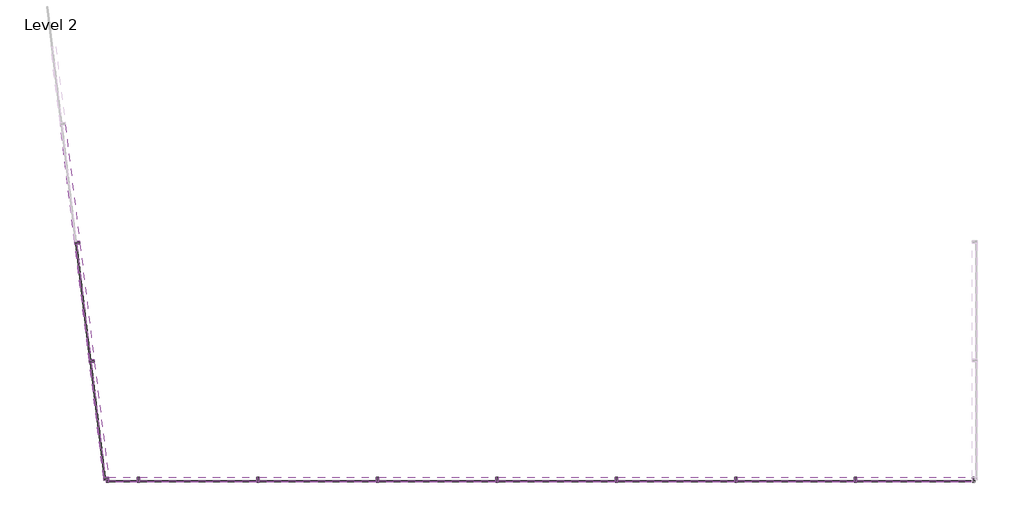
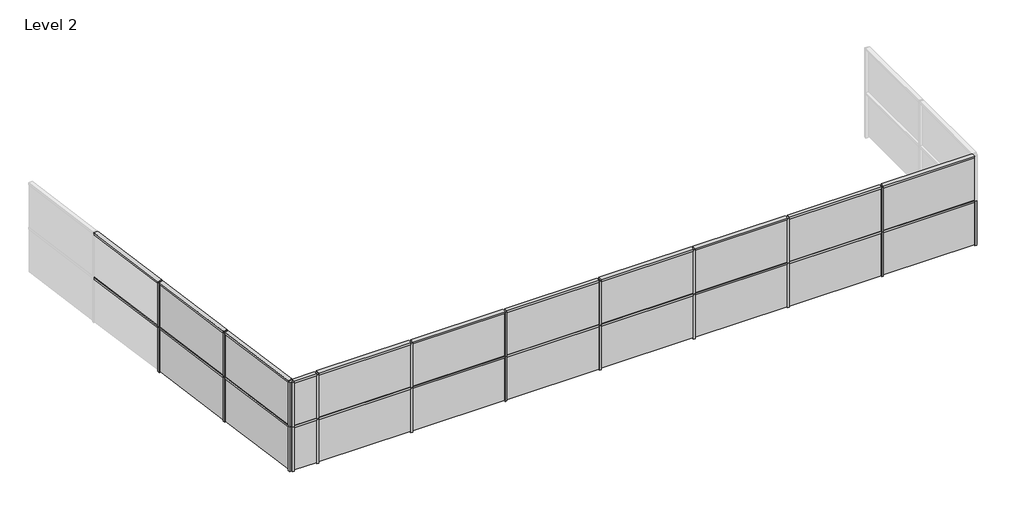
# One storey, part 1 of 2: 45 members, 20 plates.
"""IFC4 building model written with IfcOpenShell, lengths in millimetres."""

from ifc_helpers import new_model, si_unit, origin, place, context, project, spatial, transform, mapped, element, save
from components import member_19d0a4ec, member_8cef0660, member_82905deb, member_4491d118, member_0c11e56c, system_panel_glazed_e46d4b42, system_panel_glazed_2a6c68b7, system_panel_glazed_9d0e0944

model = new_model("IFC4")

# Units and contexts
model_context = context("Model", 3, world=origin())
ifc_project = project(units=[si_unit("LENGTHUNIT", "METRE", prefix="MILLI")], contexts=[model_context])

# Site, building, storey
site = spatial("IfcSite", under=ifc_project)
building = spatial("IfcBuilding", under=site)
storey = spatial("IfcBuildingStorey", under=building, Name="Level 2", Elevation=3048.0)

# Members
placement = place(None, origin())
member_shape = member_19d0a4ec(model_context)
element("IfcMember", 1, ObjectType="Rectangular Mullion : 2.5\" x 5\" rectangular", at=placement, inside=storey, context=model_context, shape_type="MappedRepresentation", body=[
    mapped(member_shape, transform((-8260.4765148, -6916.1096898, 4572.0), x_axis=(0.0, 0.0, 1.0), y_axis=(-0.9925461516413222, -0.12186934340514591, 0.0), z_axis=(0.12186934340514591, -0.9925461516413222, 0.0))),
])
element("IfcMember", 2, ObjectType="Rectangular Mullion : 2.5\" x 5\" rectangular", at=placement, inside=storey, context=model_context, shape_type="MappedRepresentation", body=[
    mapped(member_shape, transform((-8260.4765148, -6916.1096898, 6096.0), x_axis=(0.0, 0.0, 1.0), y_axis=(-0.9925461516413222, -0.12186934340514587, 0.0), z_axis=(0.12186934340514587, -0.9925461516413222, 0.0))),
])
element("IfcMember", 3, ObjectType="Rectangular Mullion : 2.5\" x 5\" rectangular", at=placement, inside=storey, context=model_context, shape_type="MappedRepresentation", body=[
    mapped(member_shape, transform((13839.0156363, -6979.1363705, 4572.0), x_axis=(0.0, 0.0, 1.0), y_axis=(0.0, -1.0, 0.0), z_axis=(1.0, 0.0, 0.0))),
])
element("IfcMember", 4, ObjectType="Rectangular Mullion : 2.5\" x 5\" rectangular", at=placement, inside=storey, context=model_context, shape_type="MappedRepresentation", body=[
    mapped(member_shape, transform((13839.0156363, -6979.1363705, 6096.0), x_axis=(0.0, 0.0, 1.0), y_axis=(0.0, -1.0, 0.0), z_axis=(1.0, 0.0, 0.0))),
])
member_2_shape = member_8cef0660(model_context)
element("IfcMember", 5, ObjectType="Rectangular Mullion : 2.5\" x 5\" rectangular", at=placement, inside=storey, context=model_context, shape_type="MappedRepresentation", body=[
    mapped(member_2_shape, transform((-8628.0649219, -3922.3423596, 4572.0), x_axis=(0.0, 0.0, 1.0), y_axis=(-0.9925461516413222, -0.12186934340514596, 0.0), z_axis=(0.12186934340514596, -0.9925461516413222, 0.0))),
])
element("IfcMember", 6, ObjectType="Rectangular Mullion : 2.5\" x 5\" rectangular", at=placement, inside=storey, context=model_context, shape_type="MappedRepresentation", body=[
    mapped(member_2_shape, transform((-8999.5226806, -897.0616894, 4572.0), x_axis=(0.0, 0.0, 1.0), y_axis=(-0.9925461516413222, -0.12186934340514602, 0.0), z_axis=(0.12186934340514602, -0.9925461516413222, 0.0))),
])
element("IfcMember", 7, ObjectType="Rectangular Mullion : 2.5\" x 5\" rectangular", at=placement, inside=storey, context=model_context, shape_type="MappedRepresentation", body=[
    mapped(member_2_shape, transform((-8628.0649219, -3922.3423596, 6096.0), x_axis=(0.0, 0.0, 1.0), y_axis=(-0.9925461516413222, -0.12186934340514596, 0.0), z_axis=(0.12186934340514596, -0.9925461516413222, 0.0))),
])
element("IfcMember", 8, ObjectType="Rectangular Mullion : 2.5\" x 5\" rectangular", at=placement, inside=storey, context=model_context, shape_type="MappedRepresentation", body=[
    mapped(member_2_shape, transform((-8999.5226806, -897.0616894, 6096.0), x_axis=(0.0, 0.0, 1.0), y_axis=(-0.9925461516413222, -0.12186934340514602, 0.0), z_axis=(0.12186934340514602, -0.9925461516413222, 0.0))),
])
element("IfcMember", 9, ObjectType="Rectangular Mullion : 2.5\" x 5\" rectangular", at=placement, inside=storey, context=model_context, shape_type="MappedRepresentation", body=[
    mapped(member_2_shape, transform((10822.765636, -6979.1363705, 4572.0), x_axis=(0.0, 0.0, 1.0), y_axis=(0.0, -1.0, 0.0), z_axis=(1.0, 0.0, 0.0))),
])
element("IfcMember", 10, ObjectType="Rectangular Mullion : 2.5\" x 5\" rectangular", at=placement, inside=storey, context=model_context, shape_type="MappedRepresentation", body=[
    mapped(member_2_shape, transform((7774.765636, -6979.1363705, 4572.0), x_axis=(0.0, 0.0, 1.0), y_axis=(0.0, -1.0, 0.0), z_axis=(1.0, 0.0, 0.0))),
])
element("IfcMember", 11, ObjectType="Rectangular Mullion : 2.5\" x 5\" rectangular", at=placement, inside=storey, context=model_context, shape_type="MappedRepresentation", body=[
    mapped(member_2_shape, transform((4726.765636, -6979.1363705, 4572.0), x_axis=(0.0, 0.0, 1.0), y_axis=(0.0, -1.0, 0.0), z_axis=(1.0, 0.0, 0.0))),
])
element("IfcMember", 12, ObjectType="Rectangular Mullion : 2.5\" x 5\" rectangular", at=placement, inside=storey, context=model_context, shape_type="MappedRepresentation", body=[
    mapped(member_2_shape, transform((1678.765636, -6979.1363705, 4572.0), x_axis=(0.0, 0.0, 1.0), y_axis=(0.0, -1.0, 0.0), z_axis=(1.0, 0.0, 0.0))),
])
element("IfcMember", 13, ObjectType="Rectangular Mullion : 2.5\" x 5\" rectangular", at=placement, inside=storey, context=model_context, shape_type="MappedRepresentation", body=[
    mapped(member_2_shape, transform((-1369.234364, -6979.1363705, 4572.0), x_axis=(0.0, 0.0, 1.0), y_axis=(0.0, -1.0, 0.0), z_axis=(1.0, 0.0, 0.0))),
])
element("IfcMember", 14, ObjectType="Rectangular Mullion : 2.5\" x 5\" rectangular", at=placement, inside=storey, context=model_context, shape_type="MappedRepresentation", body=[
    mapped(member_2_shape, transform((-4417.234364, -6979.1363705, 4572.0), x_axis=(0.0, 0.0, 1.0), y_axis=(0.0, -1.0, 0.0), z_axis=(1.0, 0.0, 0.0))),
])
element("IfcMember", 15, ObjectType="Rectangular Mullion : 2.5\" x 5\" rectangular", at=placement, inside=storey, context=model_context, shape_type="MappedRepresentation", body=[
    mapped(member_2_shape, transform((10822.765636, -6979.1363705, 6096.0), x_axis=(0.0, 0.0, 1.0), y_axis=(0.0, -1.0, 0.0), z_axis=(1.0, 0.0, 0.0))),
])
element("IfcMember", 16, ObjectType="Rectangular Mullion : 2.5\" x 5\" rectangular", at=placement, inside=storey, context=model_context, shape_type="MappedRepresentation", body=[
    mapped(member_2_shape, transform((7774.765636, -6979.1363705, 6096.0), x_axis=(0.0, 0.0, 1.0), y_axis=(0.0, -1.0, 0.0), z_axis=(1.0, 0.0, 0.0))),
])
element("IfcMember", 17, ObjectType="Rectangular Mullion : 2.5\" x 5\" rectangular", at=placement, inside=storey, context=model_context, shape_type="MappedRepresentation", body=[
    mapped(member_2_shape, transform((4726.765636, -6979.1363705, 6096.0), x_axis=(0.0, 0.0, 1.0), y_axis=(0.0, -1.0, 0.0), z_axis=(1.0, 0.0, 0.0))),
])
element("IfcMember", 18, ObjectType="Rectangular Mullion : 2.5\" x 5\" rectangular", at=placement, inside=storey, context=model_context, shape_type="MappedRepresentation", body=[
    mapped(member_2_shape, transform((1678.765636, -6979.1363705, 6096.0), x_axis=(0.0, 0.0, 1.0), y_axis=(0.0, -1.0, 0.0), z_axis=(1.0, 0.0, 0.0))),
])
element("IfcMember", 19, ObjectType="Rectangular Mullion : 2.5\" x 5\" rectangular", at=placement, inside=storey, context=model_context, shape_type="MappedRepresentation", body=[
    mapped(member_2_shape, transform((-1369.234364, -6979.1363705, 6096.0), x_axis=(0.0, 0.0, 1.0), y_axis=(0.0, -1.0, 0.0), z_axis=(1.0, 0.0, 0.0))),
])
element("IfcMember", 20, ObjectType="Rectangular Mullion : 2.5\" x 5\" rectangular", at=placement, inside=storey, context=model_context, shape_type="MappedRepresentation", body=[
    mapped(member_2_shape, transform((-4417.234364, -6979.1363705, 6096.0), x_axis=(0.0, 0.0, 1.0), y_axis=(0.0, -1.0, 0.0), z_axis=(1.0, 0.0, 0.0))),
])
member_3_shape = member_82905deb(model_context)
element("IfcMember", 21, ObjectType="Rectangular Mullion : 2.5\" x 5\" rectangular", at=placement, inside=storey, context=model_context, shape_type="MappedRepresentation", body=[
    mapped(member_3_shape, transform((-8624.1955702, -3953.8557, 4572.0), x_axis=(-0.12186934340514591, 0.9925461516413222, 0.0), y_axis=(-0.9925461516413222, -0.12186934340514591, 0.0), z_axis=(0.0, 0.0, 1.0))),
])
element("IfcMember", 22, ObjectType="Rectangular Mullion : 2.5\" x 5\" rectangular", at=placement, inside=storey, context=model_context, shape_type="MappedRepresentation", body=[
    mapped(member_3_shape, transform((-8624.1955702, -3953.8557, 6096.0), x_axis=(-0.12186934340514591, 0.9925461516413222, 0.0), y_axis=(-0.9925461516413222, -0.12186934340514591, 0.0), z_axis=(0.0, 0.0, 1.0))),
])
element("IfcMember", 23, ObjectType="Rectangular Mullion : 2.5\" x 5\" rectangular", at=placement, inside=storey, context=model_context, shape_type="MappedRepresentation", body=[
    mapped(member_3_shape, transform((-8995.6533289, -928.5750297, 4572.0), x_axis=(-0.12186934340514591, 0.9925461516413222, 0.0), y_axis=(-0.9925461516413222, -0.12186934340514591, 0.0), z_axis=(0.0, 0.0, 1.0))),
])
element("IfcMember", 24, ObjectType="Rectangular Mullion : 2.5\" x 5\" rectangular", at=placement, inside=storey, context=model_context, shape_type="MappedRepresentation", body=[
    mapped(member_3_shape, transform((-8995.6533289, -928.5750297, 6096.0), x_axis=(-0.12186934340514591, 0.9925461516413222, 0.0), y_axis=(-0.9925461516413222, -0.12186934340514591, 0.0), z_axis=(0.0, 0.0, 1.0))),
])
element("IfcMember", 25, ObjectType="Rectangular Mullion : 2.5\" x 5\" rectangular", at=placement, inside=storey, context=model_context, shape_type="MappedRepresentation", body=[
    mapped(member_3_shape, transform((10854.515636, -6979.1363705, 4572.0), x_axis=(-1.0, 0.0, 0.0), y_axis=(0.0, -1.0, 0.0), z_axis=(0.0, 0.0, 1.0))),
])
element("IfcMember", 26, ObjectType="Rectangular Mullion : 2.5\" x 5\" rectangular", at=placement, inside=storey, context=model_context, shape_type="MappedRepresentation", body=[
    mapped(member_3_shape, transform((10854.515636, -6979.1363705, 6096.0), x_axis=(-1.0, 0.0, 0.0), y_axis=(0.0, -1.0, 0.0), z_axis=(0.0, 0.0, 1.0))),
])
element("IfcMember", 27, ObjectType="Rectangular Mullion : 2.5\" x 5\" rectangular", at=placement, inside=storey, context=model_context, shape_type="MappedRepresentation", body=[
    mapped(member_3_shape, transform((7806.515636, -6979.1363705, 4572.0), x_axis=(-1.0, 0.0, 0.0), y_axis=(0.0, -1.0, 0.0), z_axis=(0.0, 0.0, 1.0))),
])
element("IfcMember", 28, ObjectType="Rectangular Mullion : 2.5\" x 5\" rectangular", at=placement, inside=storey, context=model_context, shape_type="MappedRepresentation", body=[
    mapped(member_3_shape, transform((7806.515636, -6979.1363705, 6096.0), x_axis=(-1.0, 0.0, 0.0), y_axis=(0.0, -1.0, 0.0), z_axis=(0.0, 0.0, 1.0))),
])
element("IfcMember", 29, ObjectType="Rectangular Mullion : 2.5\" x 5\" rectangular", at=placement, inside=storey, context=model_context, shape_type="MappedRepresentation", body=[
    mapped(member_3_shape, transform((4758.515636, -6979.1363705, 4572.0), x_axis=(-1.0, 0.0, 0.0), y_axis=(0.0, -1.0, 0.0), z_axis=(0.0, 0.0, 1.0))),
])
element("IfcMember", 30, ObjectType="Rectangular Mullion : 2.5\" x 5\" rectangular", at=placement, inside=storey, context=model_context, shape_type="MappedRepresentation", body=[
    mapped(member_3_shape, transform((4758.515636, -6979.1363705, 6096.0), x_axis=(-1.0, 0.0, 0.0), y_axis=(0.0, -1.0, 0.0), z_axis=(0.0, 0.0, 1.0))),
])
element("IfcMember", 31, ObjectType="Rectangular Mullion : 2.5\" x 5\" rectangular", at=placement, inside=storey, context=model_context, shape_type="MappedRepresentation", body=[
    mapped(member_3_shape, transform((1710.515636, -6979.1363705, 4572.0), x_axis=(-1.0, 0.0, 0.0), y_axis=(0.0, -1.0, 0.0), z_axis=(0.0, 0.0, 1.0))),
])
element("IfcMember", 32, ObjectType="Rectangular Mullion : 2.5\" x 5\" rectangular", at=placement, inside=storey, context=model_context, shape_type="MappedRepresentation", body=[
    mapped(member_3_shape, transform((1710.515636, -6979.1363705, 6096.0), x_axis=(-1.0, 0.0, 0.0), y_axis=(0.0, -1.0, 0.0), z_axis=(0.0, 0.0, 1.0))),
])
element("IfcMember", 33, ObjectType="Rectangular Mullion : 2.5\" x 5\" rectangular", at=placement, inside=storey, context=model_context, shape_type="MappedRepresentation", body=[
    mapped(member_3_shape, transform((-1337.484364, -6979.1363705, 4572.0), x_axis=(-1.0, 0.0, 0.0), y_axis=(0.0, -1.0, 0.0), z_axis=(0.0, 0.0, 1.0))),
])
element("IfcMember", 34, ObjectType="Rectangular Mullion : 2.5\" x 5\" rectangular", at=placement, inside=storey, context=model_context, shape_type="MappedRepresentation", body=[
    mapped(member_3_shape, transform((-1337.484364, -6979.1363705, 6096.0), x_axis=(-1.0, 0.0, 0.0), y_axis=(0.0, -1.0, 0.0), z_axis=(0.0, 0.0, 1.0))),
])
element("IfcMember", 35, ObjectType="Rectangular Mullion : 2.5\" x 5\" rectangular", at=placement, inside=storey, context=model_context, shape_type="MappedRepresentation", body=[
    mapped(member_3_shape, transform((-4385.484364, -6979.1363705, 4572.0), x_axis=(-1.0, 0.0, 0.0), y_axis=(0.0, -1.0, 0.0), z_axis=(0.0, 0.0, 1.0))),
])
element("IfcMember", 36, ObjectType="Rectangular Mullion : 2.5\" x 5\" rectangular", at=placement, inside=storey, context=model_context, shape_type="MappedRepresentation", body=[
    mapped(member_3_shape, transform((-4385.484364, -6979.1363705, 6096.0), x_axis=(-1.0, 0.0, 0.0), y_axis=(0.0, -1.0, 0.0), z_axis=(0.0, 0.0, 1.0))),
])
element("IfcMember", 37, ObjectType="Rectangular Mullion : 2.5\" x 5\" rectangular", at=placement, inside=storey, context=model_context, shape_type="MappedRepresentation", body=[
    mapped(member_3_shape, transform((-7433.484364, -6979.1363705, 4572.0), x_axis=(-1.0, 0.0, 0.0), y_axis=(0.0, -1.0, 0.0), z_axis=(0.0, 0.0, 1.0))),
])
element("IfcMember", 38, ObjectType="Rectangular Mullion : 2.5\" x 5\" rectangular", at=placement, inside=storey, context=model_context, shape_type="MappedRepresentation", body=[
    mapped(member_3_shape, transform((-7433.484364, -6979.1363705, 6096.0), x_axis=(-1.0, 0.0, 0.0), y_axis=(0.0, -1.0, 0.0), z_axis=(0.0, 0.0, 1.0))),
])
member_4_shape = member_4491d118(model_context)
element("IfcMember", 39, ObjectType="Rectangular Mullion : 2.5\" x 5\" rectangular", at=placement, inside=storey, context=model_context, shape_type="MappedRepresentation", body=[
    mapped(member_4_shape, transform((-8252.7378115, -6979.1363705, 3048.0), x_axis=(0.12186934340514591, -0.9925461516413222, 0.0), y_axis=(-0.9925461516413222, -0.12186934340514591, 0.0), z_axis=(0.0, 0.0, -1.0))),
])
element("IfcMember", 40, ObjectType="Rectangular Mullion : 2.5\" x 5\" rectangular", at=placement, inside=storey, context=model_context, shape_type="MappedRepresentation", body=[
    mapped(member_4_shape, transform((-8252.7378115, -6979.1363705, 4572.0), x_axis=(0.12186934340514591, -0.9925461516413222, 0.0), y_axis=(-0.9925461516413222, -0.12186934340514591, 0.0), z_axis=(0.0, 0.0, -1.0))),
])
element("IfcMember", 41, ObjectType="Rectangular Mullion : 2.5\" x 5\" rectangular", at=placement, inside=storey, context=model_context, shape_type="MappedRepresentation", body=[
    mapped(member_4_shape, transform((13902.5156363, -6979.1363705, 3048.0), x_axis=(1.0, 0.0, 0.0), y_axis=(0.0, -1.0, 0.0), z_axis=(0.0, 0.0, -1.0))),
])
element("IfcMember", 42, ObjectType="Rectangular Mullion : 2.5\" x 5\" rectangular", at=placement, inside=storey, context=model_context, shape_type="MappedRepresentation", body=[
    mapped(member_4_shape, transform((-8252.7378115, -6979.1363705, 4572.0), x_axis=(-1.0, 0.0, 0.0), y_axis=(0.0, -1.0, 0.0), z_axis=(0.0, 0.0, 1.0))),
])
element("IfcMember", 43, ObjectType="Rectangular Mullion : 2.5\" x 5\" rectangular", at=placement, inside=storey, context=model_context, shape_type="MappedRepresentation", body=[
    mapped(member_4_shape, transform((-8252.7378115, -6979.1363705, 6096.0), x_axis=(-1.0, 0.0, 0.0), y_axis=(0.0, -1.0, 0.0), z_axis=(0.0, 0.0, 1.0))),
])
member_5_shape = member_0c11e56c(model_context)
element("IfcMember", 44, ObjectType="Rectangular Mullion : 2.5\" x 5\" rectangular", at=placement, inside=storey, context=model_context, shape_type="MappedRepresentation", body=[
    mapped(member_5_shape, transform((-7465.234364, -6979.1363705, 4572.0), x_axis=(0.0, 0.0, 1.0), y_axis=(0.0, -1.0, 0.0), z_axis=(1.0, 0.0, 0.0))),
])
element("IfcMember", 45, ObjectType="Rectangular Mullion : 2.5\" x 5\" rectangular", at=placement, inside=storey, context=model_context, shape_type="MappedRepresentation", body=[
    mapped(member_5_shape, transform((-7465.234364, -6979.1363705, 6096.0), x_axis=(0.0, 0.0, 1.0), y_axis=(0.0, -1.0, 0.0), z_axis=(1.0, 0.0, 0.0))),
])

# Plates
system_panel_glazed_shape = system_panel_glazed_e46d4b42(model_context)
element("IfcPlate", 46, ObjectType="System Panel : Glazed", at=placement, inside=storey, context=model_context, shape_type="MappedRepresentation", body=[
    mapped(system_panel_glazed_shape, transform((-8440.4013667, -5450.739365, 3079.75), x_axis=(-0.12186934340514591, 0.9925461516413222, 0.0), y_axis=(-0.9925461516413222, -0.12186934340514591, 0.0), z_axis=(0.0, 0.0, 1.0))),
])
element("IfcPlate", 47, ObjectType="System Panel : Glazed", at=placement, inside=storey, context=model_context, shape_type="MappedRepresentation", body=[
    mapped(system_panel_glazed_shape, transform((-8440.4013667, -5450.739365, 4603.75), x_axis=(-0.12186934340514591, 0.9925461516413222, 0.0), y_axis=(-0.9925461516413222, -0.12186934340514591, 0.0), z_axis=(0.0, 0.0, 1.0))),
])
element("IfcPlate", 48, ObjectType="System Panel : Glazed", at=placement, inside=storey, context=model_context, shape_type="MappedRepresentation", body=[
    mapped(system_panel_glazed_shape, transform((12362.6406361, -6979.1363705, 3079.75), x_axis=(-1.0, 0.0, 0.0), y_axis=(0.0, -1.0, 0.0), z_axis=(0.0, 0.0, 1.0))),
])
element("IfcPlate", 49, ObjectType="System Panel : Glazed", at=placement, inside=storey, context=model_context, shape_type="MappedRepresentation", body=[
    mapped(system_panel_glazed_shape, transform((12362.6406361, -6979.1363705, 4603.75), x_axis=(-1.0, 0.0, 0.0), y_axis=(0.0, -1.0, 0.0), z_axis=(0.0, 0.0, 1.0))),
])
system_panel_glazed_2_shape = system_panel_glazed_2a6c68b7(model_context)
element("IfcPlate", 50, ObjectType="System Panel : Glazed", at=placement, inside=storey, context=model_context, shape_type="MappedRepresentation", body=[
    mapped(system_panel_glazed_2_shape, transform((-8809.9244496, -2441.2153649, 3079.75), x_axis=(-0.12186934340514591, 0.9925461516413222, 0.0), y_axis=(-0.9925461516413222, -0.12186934340514591, 0.0), z_axis=(0.0, 0.0, 1.0))),
])
element("IfcPlate", 51, ObjectType="System Panel : Glazed", at=placement, inside=storey, context=model_context, shape_type="MappedRepresentation", body=[
    mapped(system_panel_glazed_2_shape, transform((-8809.9244496, -2441.2153649, 4603.75), x_axis=(-0.12186934340514591, 0.9925461516413222, 0.0), y_axis=(-0.9925461516413222, -0.12186934340514591, 0.0), z_axis=(0.0, 0.0, 1.0))),
])
element("IfcPlate", 52, ObjectType="System Panel : Glazed", at=placement, inside=storey, context=model_context, shape_type="MappedRepresentation", body=[
    mapped(system_panel_glazed_2_shape, transform((9330.515636, -6979.1363705, 3079.75), x_axis=(-1.0, 0.0, 0.0), y_axis=(0.0, -1.0, 0.0), z_axis=(0.0, 0.0, 1.0))),
])
element("IfcPlate", 53, ObjectType="System Panel : Glazed", at=placement, inside=storey, context=model_context, shape_type="MappedRepresentation", body=[
    mapped(system_panel_glazed_2_shape, transform((6282.515636, -6979.1363705, 3079.75), x_axis=(-1.0, 0.0, 0.0), y_axis=(0.0, -1.0, 0.0), z_axis=(0.0, 0.0, 1.0))),
])
element("IfcPlate", 54, ObjectType="System Panel : Glazed", at=placement, inside=storey, context=model_context, shape_type="MappedRepresentation", body=[
    mapped(system_panel_glazed_2_shape, transform((3234.515636, -6979.1363705, 3079.75), x_axis=(-1.0, 0.0, 0.0), y_axis=(0.0, -1.0, 0.0), z_axis=(0.0, 0.0, 1.0))),
])
element("IfcPlate", 55, ObjectType="System Panel : Glazed", at=placement, inside=storey, context=model_context, shape_type="MappedRepresentation", body=[
    mapped(system_panel_glazed_2_shape, transform((186.515636, -6979.1363705, 3079.75), x_axis=(-1.0, 0.0, 0.0), y_axis=(0.0, -1.0, 0.0), z_axis=(0.0, 0.0, 1.0))),
])
element("IfcPlate", 56, ObjectType="System Panel : Glazed", at=placement, inside=storey, context=model_context, shape_type="MappedRepresentation", body=[
    mapped(system_panel_glazed_2_shape, transform((-2861.484364, -6979.1363705, 3079.75), x_axis=(-1.0, 0.0, 0.0), y_axis=(0.0, -1.0, 0.0), z_axis=(0.0, 0.0, 1.0))),
])
element("IfcPlate", 57, ObjectType="System Panel : Glazed", at=placement, inside=storey, context=model_context, shape_type="MappedRepresentation", body=[
    mapped(system_panel_glazed_2_shape, transform((-5909.484364, -6979.1363705, 3079.75), x_axis=(-1.0, 0.0, 0.0), y_axis=(0.0, -1.0, 0.0), z_axis=(0.0, 0.0, 1.0))),
])
element("IfcPlate", 58, ObjectType="System Panel : Glazed", at=placement, inside=storey, context=model_context, shape_type="MappedRepresentation", body=[
    mapped(system_panel_glazed_2_shape, transform((9330.515636, -6979.1363705, 4603.75), x_axis=(-1.0, 0.0, 0.0), y_axis=(0.0, -1.0, 0.0), z_axis=(0.0, 0.0, 1.0))),
])
element("IfcPlate", 59, ObjectType="System Panel : Glazed", at=placement, inside=storey, context=model_context, shape_type="MappedRepresentation", body=[
    mapped(system_panel_glazed_2_shape, transform((6282.515636, -6979.1363705, 4603.75), x_axis=(-1.0, 0.0, 0.0), y_axis=(0.0, -1.0, 0.0), z_axis=(0.0, 0.0, 1.0))),
])
element("IfcPlate", 60, ObjectType="System Panel : Glazed", at=placement, inside=storey, context=model_context, shape_type="MappedRepresentation", body=[
    mapped(system_panel_glazed_2_shape, transform((3234.515636, -6979.1363705, 4603.75), x_axis=(-1.0, 0.0, 0.0), y_axis=(0.0, -1.0, 0.0), z_axis=(0.0, 0.0, 1.0))),
])
element("IfcPlate", 61, ObjectType="System Panel : Glazed", at=placement, inside=storey, context=model_context, shape_type="MappedRepresentation", body=[
    mapped(system_panel_glazed_2_shape, transform((186.515636, -6979.1363705, 4603.75), x_axis=(-1.0, 0.0, 0.0), y_axis=(0.0, -1.0, 0.0), z_axis=(0.0, 0.0, 1.0))),
])
element("IfcPlate", 62, ObjectType="System Panel : Glazed", at=placement, inside=storey, context=model_context, shape_type="MappedRepresentation", body=[
    mapped(system_panel_glazed_2_shape, transform((-2861.484364, -6979.1363705, 4603.75), x_axis=(-1.0, 0.0, 0.0), y_axis=(0.0, -1.0, 0.0), z_axis=(0.0, 0.0, 1.0))),
])
element("IfcPlate", 63, ObjectType="System Panel : Glazed", at=placement, inside=storey, context=model_context, shape_type="MappedRepresentation", body=[
    mapped(system_panel_glazed_2_shape, transform((-5909.484364, -6979.1363705, 4603.75), x_axis=(-1.0, 0.0, 0.0), y_axis=(0.0, -1.0, 0.0), z_axis=(0.0, 0.0, 1.0))),
])
system_panel_glazed_3_shape = system_panel_glazed_9d0e0944(model_context)
element("IfcPlate", 64, ObjectType="System Panel : Glazed", at=placement, inside=storey, context=model_context, shape_type="MappedRepresentation", body=[
    mapped(system_panel_glazed_3_shape, transform((-7827.2360878, -6979.1363705, 3079.75), x_axis=(-1.0, 0.0, 0.0), y_axis=(0.0, -1.0, 0.0), z_axis=(0.0, 0.0, 1.0))),
])
element("IfcPlate", 65, ObjectType="System Panel : Glazed", at=placement, inside=storey, context=model_context, shape_type="MappedRepresentation", body=[
    mapped(system_panel_glazed_3_shape, transform((-7827.2360878, -6979.1363705, 4603.75), x_axis=(-1.0, 0.0, 0.0), y_axis=(0.0, -1.0, 0.0), z_axis=(0.0, 0.0, 1.0))),
])

save(model, "model.ifc")

# Revit data of these elements
# Type "Rectangular Mullion : 2.5\" x 5\" rectangular"
#   built-in parameter 1007304 = 0.416667 (stored number, unit not read)
#   built-in parameter 1007301 = 0.104167 (stored number, unit not read)
#   built-in parameter 1007300 = 0.104167 (stored number, unit not read)
# Type "System Panel : Glazed"
#   Construction Type Id = "GSP4R"
#   Analytic Construction = "1/8 in Pilkington single glazing"
#   Visual Light Transmittance = 0.9
#   Solar Heat Gain Coefficient = 0.86
#   Heat Transfer Coefficient (U) = 1.18115 BTU/(h·ft²·°F)
#   Define Thermal Properties by = 1
# Elements 1, 2, 3, 4, 5, 6, 7, 8, 9, 10, 11, 12, 13, 14, 15, 16, 17, 18, 19, 20, 21, 22, 23, 24, 25, 26, 27, 28, 29, 30, 31, 32, 33, 34, 35, 36, 37, 38, 39, 40, 41, 42, 43, 44, 45 (IfcMember, "Rectangular Mullion : 2.5\" x 5\" rectangular")
#   Phase Created = New Construction
#   Materials on its faces: "Aluminum"
# Elements 46, 47, 48, 49, 50, 51, 52, 53, 54, 55, 56, 57, 58, 59, 60, 61, 62, 63, 64, 65 (IfcPlate, "System Panel : Glazed")
#   Phase Created = New Construction
#   Materials on its faces: "Glass"
# Materials
#   "Aluminum": class "Metal", colour RGB 247 247 247, transparency 0, Description = "Aluminum 6061", Cost = 0
#   "Glass": class "Glass", colour RGB 0 128 192, transparency 0.75, Description = "Soda Lime Glass", Cost = 0
